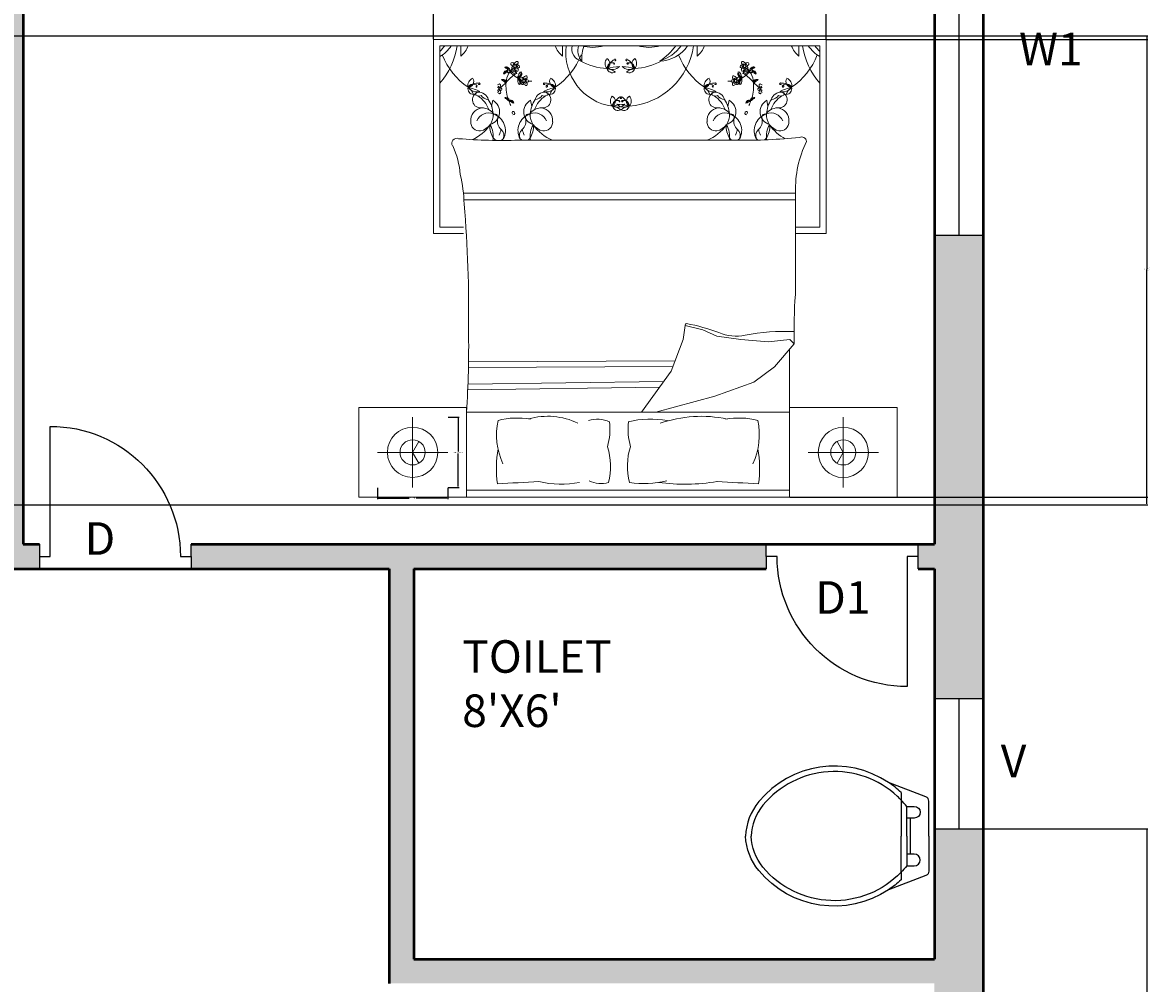
# Model space of a CAD drawing. Units: inches. Extents: x -15 to 420, y -514 to 86.
# Tile 7 of 8: x 212 to 420, y -251 to -74. Entities that reach past the tile are written whole.
import ezdxf

# ---------------------------------------------------------------- set-up
doc = ezdxf.new("R2010")
doc.units = ezdxf.units.IN
doc.header["$MEASUREMENT"] = 0
for name, color, linetype, lineweight in [('A-ANNO-DIMS', 2, 'Continuous', 18), ('A-ANNO-TEXT', 7, 'Continuous', 18), ('A-AREA-IDEN', 7, 'Continuous', 25), ('A-DOOR', 4, 'Continuous', 25), ('A-FLOR-FIXT', 9, 'Continuous', 25), ('A-FURN', 8, 'Continuous', 18), ('A-GLAZ', 41, 'Continuous', 25), ('A-WALL', 7, 'Continuous', 50), ('A-WALL-PATT', 8, 'Continuous', 13)]:
    doc.layers.add(name, color=color, linetype=linetype, lineweight=lineweight)
doc.styles.get("Standard").update_dxf_attribs({"font": 'arial.ttf'})
doc.dimstyles.get("Standard").update_dxf_attribs({"dimtxt": 0.18, "dimasz": 0.18, "dimexe": 0.18, "dimexo": 0.0625, "dimgap": 0.09, "dimtad": 0, "dimtih": 1, "dimtoh": 1, "dimdec": 0, "dimzin": 0, "dimdsep": 46, "dimlunit": 3, "dimtxsty": 'Standard', "dimcen": 0.09, "dimadec": 0, "dimazin": 0, "dimtfac": 1, "dimtdec": 0, "dimtofl": 0, "dimtmove": 0, "dimatfit": 3, "dimfxl": 1, "dimtolj": 1, "dimtzin": 0, "dimarcsym": 0})

# ---------------------------------------------------------------- blocks, each defined once
blk = doc.blocks.new('DOOR-SWING-24IN')
for p, q in [((26, 0), (26, 24)), ((2, 0), (0, 0)), ((28, 0), (26, 0))]:
    blk.add_line(p, q)
blk.add_arc((26, 0), 24, 90, 180)
blk = doc.blocks.new('WIN-W1-60IN')
for p, q in [((0, 60), (0, 0)), ((4.5, 60), (4.5, 0)), ((9, 0), (9, 60))]:
    blk.add_line(p, q)
blk = doc.blocks.new('VENT-V-24IN')
for p, q in [((0, 24), (0, 0)), ((4.5, 24), (4.5, 0)), ((9, 0), (9, 24))]:
    blk.add_line(p, q)
blk = doc.blocks.new('WC-PLAN')
for p, q in [((28.69, 20.98), (28.69, 19.56)), ((28.69, 19.56), (28.69, 12.91)), ((28.69, 6.26), (28.69, 12.91)), ((28.69, 6.26), (28.69, 4.85))]:
    blk.add_line(p, q)
for points in [[(26.37, 22.81, 0.383919), (2.44, 19.27, 0.163732), (0, 12.91, 0.359733)], [(28, 20.24, 0.431639), (3.21, 18.62, 0.162618), (1.01, 12.91, 0.470877)], [(28.69, 20.98, 0.040937), (26.37, 22.81, 0.163732)], [(33.8, 12.91), (33.8, 19.37, 0.31031), (33.26, 20.16), (26.37, 22.81, 0.209071)], [(28.69, 19.56, 0.014165), (28, 20.24, 0.162618)], [(29.71, 18.4, 0.022712), (28.69, 19.56, 0.162618)], [(29.71, 12.91), (29.71, 18.4, 0.022712)], [(29.71, 18.4), (31.12, 18.4, -1), (31.12, 16.24), (30.39, 16.24)], [(26.37, 3.02, -0.383919), (2.44, 6.56, -0.163732), (0, 12.91, -0.359733)], [(28.69, 6.26, -0.448546), (3.21, 7.2, -0.162618), (1.01, 12.91, -0.470877)], [(33.8, 12.91), (33.8, 6.46, -0.31031), (33.26, 5.67), (26.37, 3.02, -0.209071)], [(29.71, 12.91), (29.71, 7.43, -0.476108)], [(29.71, 7.43), (31.12, 7.43, 1), (31.12, 9.59), (30.39, 9.59)], [(29.71, 7.43, -0.022712), (28.69, 6.26, -0.162618)], [(28.69, 4.85, -0.040937), (26.37, 3.02, -0.163732)]]:
    blk.add_lwpolyline(points, format="xyb")
for points in [[(30.39, 16.24), (29.71, 16.24)], [(30.39, 9.59), (30.39, 16.24)], [(30.39, 9.59), (29.71, 9.59)]]:
    blk.add_lwpolyline(points)
blk = doc.blocks.new('BEDSIDE-LAMP-9-25IN')
for p, q in [((6.49, 12.97), (6.49, 0)), ((12.97, 6.49), (0, 6.49))]:
    blk.add_line(p, q)
for points in [[(6.49, 6.49), (7.64, 8.49)], [(6.49, 6.49), (7.64, 4.48)]]:
    blk.add_lwpolyline(points)
for radius in [4.63, 2.32]:
    blk.add_circle((6.49, 6.49), radius)
blk = doc.blocks.new('*D37')
at = {"layer": 'A-ANNO-DIMS', "color": 0, "lineweight": -2, "transparency": 16777216}
for p, q in [((290.77, -146.45), (292.83, -146.45)), ((292.65, -146.63), (292.65, -152.75)), ((292.65, -159.24), (292.65, -153.11)), ((290.77, -159.42), (292.83, -159.42))]:
    blk.add_line(p, q, dxfattribs=at)
at = {"layer": 'A-ANNO-DIMS', "color": 0, "transparency": 16777216}
for points in [[(292.62, -146.63), (292.68, -146.63), (292.65, -146.45)], [(292.62, -159.24), (292.68, -159.24), (292.65, -159.42)]]:
    blk.add_solid(points, dxfattribs=at)
at = {"layer": 'Defpoints', "color": 0, "transparency": 16777216}
for p in [(290.7, -146.45), (292.65, -146.45), (290.7, -159.42)]:
    blk.add_point(p, dxfattribs=at)
at = {"layer": 'A-ANNO-DIMS', "color": 0, "transparency": 16777216, "insert": (292.65, -152.93), "char_height": 0.18, "attachment_point": 5}
blk.add_mtext('\\A1;LAMP 1\'-1" TYP.', dxfattribs=at)
blk = doc.blocks.new('*D38')
at = {"layer": 'A-ANNO-DIMS', "color": 0, "lineweight": -2, "transparency": 16777216}
for p, q in [((277.73, -159.48), (277.73, -161.55)), ((290.7, -159.48), (290.7, -161.55)), ((277.91, -161.37), (283.59, -161.37)), ((290.52, -161.37), (284.85, -161.37))]:
    blk.add_line(p, q, dxfattribs=at)
at = {"layer": 'A-ANNO-DIMS', "color": 0, "transparency": 16777216}
for points in [[(277.91, -161.34), (277.91, -161.4), (277.73, -161.37)], [(290.52, -161.34), (290.52, -161.4), (290.7, -161.37)]]:
    blk.add_solid(points, dxfattribs=at)
at = {"layer": 'Defpoints', "color": 0, "transparency": 16777216}
for p in [(277.73, -159.42), (290.7, -159.42), (290.7, -161.37)]:
    blk.add_point(p, dxfattribs=at)
at = {"layer": 'A-ANNO-DIMS', "color": 0, "transparency": 16777216, "insert": (284.22, -161.37), "char_height": 0.18, "attachment_point": 5}
blk.add_mtext('\\A1;1\'-1" TYP.', dxfattribs=at)
blk = doc.blocks.new('*D62')
at = {"layer": 'A-ANNO-DIMS', "color": 0, "lineweight": -2, "transparency": 16777216}
for p, q in [((389.49, -222.38), (419.8, -222.38)), ((419.62, -222.56), (419.62, -272.45)), ((419.62, -322.7), (419.62, -272.81)), ((389.49, -322.88), (419.8, -322.88))]:
    blk.add_line(p, q, dxfattribs=at)
at = {"layer": 'A-ANNO-DIMS', "color": 0, "transparency": 16777216}
for points in [[(419.59, -222.56), (419.65, -222.56), (419.62, -222.38)], [(419.59, -322.7), (419.65, -322.7), (419.62, -322.88)]]:
    blk.add_solid(points, dxfattribs=at)
at = {"layer": 'Defpoints', "color": 0, "transparency": 16777216}
for p in [(389.42, -222.38), (419.62, -222.38), (389.42, -322.88)]:
    blk.add_point(p, dxfattribs=at)
at = {"layer": 'A-ANNO-DIMS', "color": 0, "transparency": 16777216, "insert": (419.62, -272.63), "char_height": 0.18, "attachment_point": 5}
blk.add_mtext('\\A1;8\'-4 1/2"', dxfattribs=at)
blk = doc.blocks.new('*D69')
at = {"layer": 'A-ANNO-DIMS', "color": 0, "lineweight": -2, "transparency": 16777216}
for p, q in [((141.76, -76.1), (419.8, -76.1)), ((419.62, -76.28), (419.62, -119.16)), ((419.62, -162.4), (419.62, -119.53)), ((134.84, -162.58), (419.8, -162.58))]:
    blk.add_line(p, q, dxfattribs=at)
at = {"layer": 'A-ANNO-DIMS', "color": 0, "transparency": 16777216}
for points in [[(419.59, -76.28), (419.65, -76.28), (419.62, -76.1)], [(419.59, -162.4), (419.65, -162.4), (419.62, -162.58)]]:
    blk.add_solid(points, dxfattribs=at)
at = {"layer": 'Defpoints', "color": 0, "transparency": 16777216}
for p in [(141.69, -76.1), (134.78, -162.58), (419.62, -162.58)]:
    blk.add_point(p, dxfattribs=at)
at = {"layer": 'A-ANNO-DIMS', "color": 0, "transparency": 16777216, "insert": (419.62, -119.34), "char_height": 0.18, "attachment_point": 5}
blk.add_mtext('\\A1;7\'-2 1/2"', dxfattribs=at)
blk = doc.blocks.new('*D70')
at = {"layer": 'A-ANNO-DIMS', "color": 0, "lineweight": -2, "transparency": 16777216}
for p, q in [((288.09, -76.72), (288.09, 43.5)), ((288.27, 43.32), (323.74, 43.32)), ((360.28, 43.32), (324.81, 43.32)), ((360.46, -76.72), (360.46, 43.5))]:
    blk.add_line(p, q, dxfattribs=at)
at = {"layer": 'A-ANNO-DIMS', "color": 0, "transparency": 16777216}
for points in [[(288.27, 43.35), (288.27, 43.29), (288.09, 43.32)], [(360.28, 43.35), (360.28, 43.29), (360.46, 43.32)]]:
    blk.add_solid(points, dxfattribs=at)
at = {"layer": 'Defpoints', "color": 0, "transparency": 16777216}
for p in [(360.46, 43.32), (288.09, -76.78), (360.46, -76.78)]:
    blk.add_point(p, dxfattribs=at)
at = {"layer": 'A-ANNO-DIMS', "color": 0, "transparency": 16777216, "insert": (324.27, 43.32), "char_height": 0.18, "attachment_point": 5}
blk.add_mtext('\\A1;6\'-0 1/2"', dxfattribs=at)
blk = doc.blocks.new('*D71')
at = {"layer": 'A-ANNO-DIMS', "color": 0, "lineweight": -2, "transparency": 16777216}
for p, q in [((360.53, -76.78), (419.8, -76.78)), ((419.62, -76.96), (419.62, -118.81)), ((419.62, -161.03), (419.62, -119.18)), ((353.77, -161.21), (419.8, -161.21))]:
    blk.add_line(p, q, dxfattribs=at)
at = {"layer": 'A-ANNO-DIMS', "color": 0, "transparency": 16777216}
for points in [[(419.59, -76.96), (419.65, -76.96), (419.62, -76.78)], [(419.59, -161.03), (419.65, -161.03), (419.62, -161.21)]]:
    blk.add_solid(points, dxfattribs=at)
at = {"layer": 'Defpoints', "color": 0, "transparency": 16777216}
for p in [(360.46, -76.78), (353.71, -161.21), (419.62, -161.21)]:
    blk.add_point(p, dxfattribs=at)
at = {"layer": 'A-ANNO-DIMS', "color": 0, "transparency": 16777216, "insert": (419.62, -118.99), "char_height": 0.18, "attachment_point": 5}
blk.add_mtext('\\A1;7\'-0 1/2"', dxfattribs=at)

msp = doc.modelspace()

# ---------------------------------------------------------------- hatches: boundary and pattern name
at = {"layer": 'A-WALL-PATT'}
h = msp.add_hatch(color=256, dxfattribs=at)
h.dxf.hatch_style = 1
h.paths.add_polyline_path([(266.67, -454.88), (240.92, -454.88), (240.92, -330.38), (236.42, -330.38), (236.42, -454.88), (218.42, -454.88), (218.42, -463.88), (266.67, -463.88)])
h.paths.add_polyline_path([(158.42, -454.88), (140.42, -454.88), (140.42, -394.88), (135.92, -394.88), (135.92, -454.88), (39.92, -454.88), (39.92, -412.88), (30.92, -412.88), (30.92, -463.88), (158.42, -463.88)])
h.paths.add_polyline_path([(39.92, -334.88), (135.92, -334.88), (135.92, -357.15), (140.42, -357.15), (140.42, -334.88), (173.95, -334.88), (173.95, -330.38), (39.92, -330.38), (39.92, -250.88), (155.51, -250.88), (155.51, -246.38), (140.42, -246.38), (140.42, -205.38), (138.17, -205.38), (135.92, -205.38), (135.92, -246.38), (39.92, -246.38), (39.92, -222.38), (30.92, -222.38), (30.92, -376.88), (39.92, -376.88)])
h.paths.add_polyline_path([(389.42, -382.88), (380.42, -382.88), (380.42, -454.88), (380.42, -463.88), (389.42, -463.88)])
h.paths.add_polyline_path([(352.42, -459.38), (352.42, -454.88), (326.67, -454.88), (326.67, -463.88), (352.42, -463.88)])
h.paths.add_polyline_path([(176.92, -169.88), (39.92, -169.88), (39.92, -112.88), (30.92, -112.88), (30.92, -198.38), (39.92, -198.38), (39.92, -174.38), (135.92, -174.38), (135.92, -177.38), (140.42, -177.38), (140.42, -174.38), (176.92, -174.38), (176.92, -172.13)])
h.paths.add_polyline_path([(39.92, 4.12), (93.92, 4.12), (93.92, 13.12), (30.92, 13.12), (30.92, -52.88), (39.92, -52.88)])
h.paths.add_polyline_path([(266.42, 13.12), (153.92, 13.12), (153.92, 4.12), (207.92, 4.12), (207.92, -169.88), (204.92, -169.88), (204.92, -174.38), (215.42, -174.38), (215.42, -169.88), (212.42, -169.88), (212.42, 4.12), (266.42, 4.12)])
h.paths.add_polyline_path([(389.42, 13.12), (326.42, 13.12), (326.42, 4.12), (380.42, 4.12), (380.42, -52.88), (389.42, -52.88)])
h.paths.add_polyline_path([(389.42, -112.88), (380.42, -112.88), (380.42, -169.88), (377.42, -169.88), (377.42, -174.38), (380.42, -174.38), (380.42, -198.38), (389.42, -198.38)])
h.paths.add_polyline_path([(349.42, -172.13), (349.42, -169.88), (243.42, -169.88), (243.42, -172.13), (243.42, -174.38), (279.92, -174.38), (279.92, -250.88), (380.42, -250.88), (380.42, -322.88), (389.42, -322.88), (389.42, -222.38), (380.42, -222.38), (380.42, -246.38), (284.42, -246.38), (284.42, -174.38), (349.42, -174.38)])

# ---------------------------------------------------------------- linework, layer by layer
at = {"layer": 'A-DOOR'}
for p, q in [((215.42, -169.88), (215.42, -174.38)), ((243.42, -172.13), (243.42, -169.88)), ((349.42, -172.13), (349.42, -169.88)), ((377.42, -174.38), (377.42, -169.88)), ((243.42, -172.13), (243.42, -174.38)), ((349.42, -172.13), (349.42, -174.38))]:
    msp.add_line(p, q, dxfattribs=at)
at = {"layer": 'A-FURN'}
for p, q in [((288.09, -76.78), (360.46, -76.78)), ((288.09, -112.54), (288.09, -76.78)), ((360.46, -76.78), (360.46, -112.54)), ((289.24, -77.93), (289.24, -111.39)), ((359.31, -77.93), (289.24, -77.93)), ((359.31, -111.39), (359.31, -77.93)), ((299.02, -88), (298.8, -89.12)), ((305.96, -88), (306.18, -89.12)), ((342.59, -88), (342.37, -89.12)), ((349.53, -88), (349.75, -89.12)), ((303.77, -95.36), (344.08, -95.36)), ((293.6, -105.11), (354.85, -105.11)), ((293.7, -106.35), (354.85, -106.35)), ((289.24, -111.39), (293.61, -111.39)), ((354.85, -111.39), (359.31, -111.39)), ((293.59, -112.54), (288.09, -112.54)), ((360.46, -112.54), (354.85, -112.54)), ((334.09, -132.12), (334.49, -129.51)), ((334.49, -129.51), (337.71, -130.31)), ((337.71, -130.31), (340.32, -131.52)), ((331.88, -137.95), (334.09, -132.12)), ((340.32, -131.52), (344.75, -132.12)), ((344.75, -132.12), (349.77, -132.52)), ((349.77, -132.52), (353.8, -132.12)), ((354.6, -132.92), (350.98, -137.14)), ((353.8, -132.12), (354.6, -132.92)), ((353.71, -161.21), (353.71, -133.96)), ((294.5, -136.23), (332.59, -136.07)), ((294.5, -137.25), (332.2, -137.1)), ((326.44, -145.52), (331.88, -137.95)), ((350.98, -137.14), (347.16, -139.96)), ((294.41, -141.39), (329.76, -140.9)), ((294.45, -140.38), (330.5, -139.87)), ((347.16, -139.96), (339.92, -142.57)), ((339.92, -142.57), (329.1, -145.52)), ((353.71, -145.52), (294.15, -145.52)), ((294.15, -159.93), (353.71, -159.93)), ((373.57, -161.21), (274.29, -161.21))]:
    msp.add_line(p, q, dxfattribs=at)
for points in [[(293.72, -107.13, 0.056112), (293, -101.67, 0.095341), (291.61, -96.41)], [(354.81, -123.83, 0.001242), (354.85, -105, -0.127202), (356.85, -95.61)], [(299.85, -158.73, -0.074897), (299.97, -152.25, 0.472817)], [(320.15, -151.89, -0.14099), (320.35, -158.5, -0.235245)], [(324.39, -151.89, 0.14099), (324.2, -158.5, 0.235245)], [(348.01, -158.73, 0.074897), (347.89, -152.25, -0.472817)]]:
    msp.add_lwpolyline(points, format="xyb", dxfattribs=at)
for points in [[(294.15, -161.21), (294.15, -144.66), (274.29, -144.66), (274.29, -161.21)], [(353.71, -144.66), (373.57, -144.66), (373.57, -161.21)]]:
    msp.add_lwpolyline(points, dxfattribs=at)
for centre in [(303.1, -81.73), (345.45, -81.73), (304.76, -84.4), (343.79, -84.4)]:
    msp.add_circle(centre, 0.253, dxfattribs=at)
for centre, radius, start, end in [((286.09, -74.45), 6.32, 299.8884, 326.5383), ((283.82, -73.27), 7.87, 313.5186, 323.6964), ((279.59, -76.18), 12.96, 318.1144, 352.255), ((289.63, -75.91), 5.27, 311.0454, 337.4453), ((275.19, -78.74), 17.94, 356.3481, 2.5919), ((315.35, -75.91), 5.27, 202.5547, 228.9546), ((329.79, -78.74), 17.94, 177.4081, 183.6519), ((322.5, -79.18), 10.03, 172.8636, 261.8197), ((315.88, -78.48), 2.33, 166.3898, 259.0739), ((317.63, -78.8), 2.94, 162.8609, 221.9049), ((317.47, -71.11), 7.13, 252.9798, 286.4569), ((321.21, -80.09), 5.8, 158.117, 186.6195), ((320.29, -67.44), 10.54, 264.3643, 265.6213), ((325.84, -60.22), 18.84, 250.0972, 250.2783), ((323.16, -76.18), 12.96, 274.4623, 352.255), ((327.77, -71.11), 7.13, 253.5431, 287.0202), ((324.95, -67.44), 10.54, 274.3787, 275.6357), ((319.4, -60.22), 18.84, 289.7217, 289.9028), ((329.66, -74.45), 6.32, 271.272, 326.5383), ((323.25, -71.06), 11.71, 304.0123, 324.053), ((327.39, -73.27), 7.87, 287.8504, 323.6964), ((318.76, -78.74), 17.94, 356.3481, 2.5919), ((333.2, -75.91), 5.27, 311.0454, 337.4453), ((358.92, -75.91), 5.27, 202.5547, 228.9546), ((373.36, -78.74), 17.94, 177.4081, 183.6519), ((368.96, -76.18), 12.96, 187.745, 221.8856), ((362.46, -74.45), 6.32, 213.4617, 240.1116), ((364.73, -73.27), 7.87, 216.3036, 226.4814), ((301.77, -74.9), 12.96, 201.4092, 235.6135), ((303.45, -81.27), 0.417, 100.9597, 208.7804), ((303.09, -81.04), 0.588, 291.6382, 4.947), ((303.49, -81.01), 0.194, 4.947, 127.5263), ((303.21, -74.9), 12.96, 304.3865, 338.5908), ((321.09, -69.24), 12.96, 242.5854, 265.5377), ((321.15, -81.2), 1.44, 140.8855, 222.2127), ((319.51, -81.24), 1.08, 301.6373, 61.4609), ((323.18, -83.23), 3.28, 121.989, 161.0841), ((321.53, -80.58), 0.161, 288.4408, 121.989), ((321.56, -80.66), 0.0782, 171.9833, 288.4408), ((323.71, -80.58), 0.161, 58.011, 251.5592), ((323.68, -80.66), 0.0782, 251.5592, 8.0167), ((322.06, -83.23), 3.28, 18.9159, 58.011), ((325.73, -81.24), 1.08, 118.5391, 238.3627), ((324.09, -81.2), 1.44, 317.7873, 39.1145), ((324.15, -69.24), 12.96, 274.4623, 297.4146), ((345.34, -74.9), 12.96, 201.4092, 235.6135), ((345.06, -81.01), 0.194, 52.4737, 175.053), ((345.46, -81.04), 0.588, 175.053, 248.3618), ((345.1, -81.27), 0.417, 331.2196, 79.0403), ((346.78, -74.9), 12.96, 304.3865, 338.5908), ((301.26, -83.03), 0.282, 123.0979, 213.1364), ((301.75, -83.43), 0.764, 92.3172, 160.5201), ((305.24, -89.24), 7.39, 121.1156, 124.8118), ((301.66, -83.15), 0.658, 82.6008, 147.1845), ((301.47, -82.1), 0.282, 55.6077, 145.6462), ((301.28, -82.71), 0.764, 21.7087, 93.0299), ((297.25, -88.16), 7.39, 53.6254, 57.3216), ((301.58, -83.17), 0.292, 45.7354, 121.1156), ((305.56, -85.03), 4.12, 150.7959, 175.244), ((311.49, -93.81), 13.56, 127.8256, 137.7588), ((301.51, -82.52), 0.658, 342.8042, 79.6943), ((301.46, -82.45), 0.292, 338.2452, 53.6254), ((301.93, -82.64), 0.221, 158.2452, 340.6395), ((301.93, -82.8), 0.221, 225.7354, 48.1297), ((306.08, -80.79), 4.4, 201.7087, 206.2181), ((302.58, -83.8), 1.15, 40.9365, 112.7695), ((302.2, -83.41), 0.678, 49.3812, 95.5456), ((305.56, -85.03), 4.12, 137.5083, 145.9967), ((302.69, -83.15), 0.7, 61.1838, 141.6792), ((305.98, -79.56), 4.94, 220.182, 239.456), ((302.57, -81.26), 0.25, 134.3732, 211.9501), ((303.03, -80.97), 0.797, 211.9501, 255.2442), ((302.59, -81.54), 0.499, 8.5614, 112.5914), ((302.82, -82.08), 0.345, 88.5719, 233.8954), ((302.78, -82.18), 0.248, 228.2946, 6.2474), ((303.17, -82.28), 0.815, 229.3812, 289.9959), ((302.73, -81.52), 0.167, 352.868, 97.094), ((302.55, -81.88), 0.348, 298.8493, 359.9355), ((302.63, -82.18), 0.398, 4.2123, 48.1587), ((303.45, -82.12), 0.422, 183.635, 258.4363), ((302.64, -83.27), 0.837, 15.6484, 62.2957), ((303.4, -81.97), 0.241, 178.1325, 268.8919), ((303.9, -81.82), 0.768, 132.3896, 156.5724), ((303.56, -81.92), 0.414, 42.3208, 130.2111), ((303.65, -81.49), 0.523, 226.3462, 279.6513), ((303.11, -82.46), 0.608, 7.4968, 71.2737), ((303.55, -80.94), 0.828, 254.2829, 276.9148), ((303.53, -82.43), 0.195, 215.0752, 14.7644), ((303.12, -82.73), 1.15, 287.889, 359.722), ((303.7, -81.79), 0.218, 279.6513, 42.3208), ((304.56, -83.5), 0.815, 110.6625, 171.2773), ((303.51, -83.09), 0.837, 338.3627, 25.0101), ((321.14, -82.12), 1.06, 76.148, 182.2415), ((322.8, -90.82), 9.07, 92.7418, 107.407), ((320.93, -80.3), 2.05, 245.6899, 314.4589), ((320.03, -84.38), 2.21, 44.6273, 88.5415), ((321.11, -81.86), 1.07, 196.1963, 296.9726), ((321.38, -81.28), 0.0845, 140.1909, 76.0209), ((322.44, -90.82), 9.07, 72.593, 87.2582), ((324.31, -80.3), 2.05, 225.5411, 294.3101), ((325.21, -84.38), 2.21, 91.4585, 135.3727), ((324.13, -81.86), 1.07, 243.0274, 343.8037), ((323.88, -81.23), 0.14, 103.852, 39.9245), ((324.1, -82.12), 1.06, 357.7585, 103.852), ((345.04, -83.09), 0.837, 154.9899, 201.6373), ((345.43, -82.73), 1.15, 180.278, 252.111), ((343.99, -83.5), 0.815, 8.7227, 69.3375), ((344.85, -81.79), 0.218, 137.6792, 260.3487), ((344.99, -81.92), 0.414, 49.7889, 137.6792), ((344.9, -81.49), 0.523, 260.3487, 313.6538), ((345.44, -82.46), 0.608, 108.7263, 172.5032), ((345.02, -82.43), 0.195, 165.2356, 324.9248), ((345, -80.94), 0.828, 263.0852, 285.7171), ((342.57, -79.56), 4.94, 300.544, 319.818), ((345.91, -83.27), 0.837, 117.7043, 164.3516), ((345.97, -83.8), 1.15, 67.2305, 139.0635), ((345.38, -82.28), 0.815, 250.0041, 310.6188), ((345.15, -81.97), 0.241, 271.1081, 1.8675), ((344.65, -81.82), 0.768, 23.4276, 47.6104), ((345.1, -82.12), 0.422, 281.5637, 356.365), ((337.06, -93.81), 13.56, 42.2412, 52.1744), ((345.96, -81.54), 0.499, 67.4086, 171.4386), ((345.92, -82.18), 0.398, 131.8413, 175.7877), ((345.76, -82.18), 0.248, 173.7526, 311.7054), ((345.86, -83.15), 0.7, 38.3208, 118.8162), ((345.82, -81.52), 0.167, 82.906, 187.132), ((346, -81.88), 0.348, 180.0645, 241.1507), ((345.52, -80.97), 0.797, 284.7558, 328.0499), ((345.73, -82.08), 0.345, 306.1046, 91.4281), ((346.35, -83.41), 0.678, 84.4544, 130.6188), ((342.99, -85.03), 4.12, 34.0033, 42.4917), ((345.98, -81.26), 0.25, 328.0499, 45.6268), ((347.04, -82.52), 0.658, 100.3057, 197.1958), ((346.61, -82.8), 0.221, 131.8703, 314.2646), ((346.62, -82.64), 0.221, 199.3605, 21.7548), ((342.47, -80.79), 4.4, 333.7819, 338.2913), ((347.27, -82.71), 0.764, 86.9701, 158.2913), ((342.99, -85.03), 4.12, 4.756, 29.2041), ((346.97, -83.17), 0.292, 58.8844, 134.2646), ((347.09, -82.45), 0.292, 126.3746, 201.7548), ((346.89, -83.15), 0.658, 32.8155, 97.3992), ((346.8, -83.43), 0.764, 19.4799, 87.6828), ((347.08, -82.1), 0.282, 34.3538, 124.3923), ((351.3, -88.16), 7.39, 122.6784, 126.3746), ((343.31, -89.24), 7.39, 55.1882, 58.8844), ((347.29, -83.03), 0.282, 326.8636, 56.9021), ((295.85, -85.29), 1.44, 110.9613, 192.2885), ((294.41, -84.52), 1.08, 271.7131, 31.5367), ((296.6, -88.07), 3.28, 92.0648, 131.1598), ((295.38, -86.09), 1.06, 46.2238, 152.3173), ((296.47, -85.03), 0.0782, 142.0591, 258.5166), ((296.49, -84.95), 0.161, 258.5166, 92.0648), ((300.2, -85.43), 0.417, 100.9597, 142.2379), ((299.85, -85.21), 0.588, 291.6382, 4.947), ((300.24, -85.18), 0.194, 4.947, 127.5263), ((294.58, -78.24), 9.43, 307.9541, 316.8459), ((300.7, -86.96), 2.8, 82.8698, 91.6736), ((301.09, -83.94), 0.521, 205.5379, 258.6744), ((300.34, -85.71), 1.57, 59.344, 79.7412), ((300, -85.7), 1.6, 43.6929, 51.7899), ((300.98, -84.66), 0.476, 355.7131, 81.6568), ((300.71, -85.07), 0.832, 27.3659, 59.344), ((301.34, -84.52), 0.202, 202.5583, 304.2343), ((309.66, -85.24), 8.22, 176.1723, 196.4158), ((303.08, -83.27), 0.678, 305.1128, 351.2773), ((303.44, -84.52), 0.7, 3.8774, 87.1501), ((302.94, -84.24), 0.678, 352.0748, 38.2393), ((302.82, -84.77), 1.15, 343.6301, 55.4631), ((304.42, -84.45), 0.815, 172.0748, 232.6895), ((303.64, -83.15), 0.7, 271.4625, 339.4747), ((303.3, -84.54), 0.837, 318.342, 4.9894), ((304.22, -83.92), 0.25, 134.3732, 211.9501), ((305.98, -79.56), 4.94, 246.1523, 246.9499), ((304.69, -83.63), 0.797, 211.9501, 255.2442), ((304.24, -84.21), 0.499, 8.5614, 112.5914), ((304.48, -84.75), 0.345, 88.5719, 233.8954), ((304.44, -84.84), 0.248, 228.2946, 6.2474), ((304.38, -84.18), 0.167, 352.868, 97.094), ((304.21, -84.55), 0.348, 298.8493, 359.9355), ((304.29, -84.85), 0.398, 4.2123, 48.1587), ((305.1, -83.93), 0.417, 100.9597, 208.7804), ((305.11, -84.79), 0.422, 183.635, 258.4363), ((305.05, -84.64), 0.241, 178.1325, 268.8919), ((305.55, -84.49), 0.768, 132.3896, 156.5724), ((305.21, -84.58), 0.414, 42.3208, 130.2111), ((305.31, -84.15), 0.523, 226.3462, 279.6513), ((304.75, -83.71), 0.588, 291.6382, 4.947), ((304.77, -85.12), 0.608, 7.4968, 71.2737), ((305.21, -83.61), 0.828, 254.2829, 276.9148), ((305.14, -83.67), 0.194, 4.947, 127.5263), ((305.18, -85.09), 0.195, 215.0752, 14.7644), ((305.36, -84.45), 0.218, 279.6513, 42.3208), ((305.98, -79.56), 4.94, 265.2415, 272.8929), ((308.49, -84.95), 0.161, 87.9352, 281.4834), ((308.38, -88.07), 3.28, 48.8402, 87.9352), ((308.51, -85.03), 0.0782, 281.4834, 37.9409), ((309.6, -86.09), 1.06, 27.6827, 133.7762), ((310.57, -84.52), 1.08, 148.4633, 268.2869), ((309.13, -85.29), 1.44, 347.7115, 69.0387), ((339.42, -85.29), 1.44, 110.9613, 192.2885), ((337.98, -84.52), 1.08, 271.7131, 31.5367), ((340.17, -88.07), 3.28, 92.0648, 131.1598), ((338.95, -86.09), 1.06, 46.2238, 152.3173), ((340.04, -85.03), 0.0782, 142.0591, 258.5166), ((340.06, -84.95), 0.161, 258.5166, 92.0648), ((342.57, -79.56), 4.94, 267.1071, 274.7585), ((343.19, -84.45), 0.218, 137.6792, 260.3487), ((343.34, -84.58), 0.414, 49.7889, 137.6792), ((343.24, -84.15), 0.523, 260.3487, 313.6538), ((343.37, -85.09), 0.195, 165.2356, 324.9248), ((343.78, -85.12), 0.608, 108.7263, 172.5032), ((343.41, -83.67), 0.194, 52.4737, 175.053), ((343.8, -83.71), 0.588, 175.053, 248.3618), ((343.34, -83.61), 0.828, 263.0852, 285.7171), ((343.5, -84.64), 0.241, 271.1081, 1.8675), ((343, -84.49), 0.768, 23.4276, 47.6104), ((343.45, -83.93), 0.417, 331.2196, 79.0403), ((343.44, -84.79), 0.422, 281.5637, 356.365), ((344.31, -84.21), 0.499, 67.4086, 171.4386), ((344.11, -84.84), 0.248, 173.7526, 311.7054), ((344.26, -84.85), 0.398, 131.8413, 175.7877), ((344.17, -84.18), 0.167, 82.906, 187.132), ((344.34, -84.55), 0.348, 180.0645, 241.1507), ((343.86, -83.63), 0.797, 284.7558, 328.0499), ((344.07, -84.75), 0.345, 306.1046, 91.4281), ((344.91, -83.15), 0.7, 200.5253, 268.5375), ((345.11, -84.52), 0.7, 92.8499, 176.1226), ((345.25, -84.54), 0.837, 175.0106, 221.658), ((344.33, -83.92), 0.25, 328.0499, 45.6268), ((342.57, -79.56), 4.94, 293.0501, 293.8477), ((345.73, -84.77), 1.15, 124.5369, 196.3699), ((344.13, -84.45), 0.815, 307.3105, 7.9252), ((345.47, -83.27), 0.678, 188.7227, 234.8872), ((345.61, -84.24), 0.678, 141.7607, 187.9252), ((338.89, -85.24), 8.22, 343.5842, 3.8277), ((347.57, -84.66), 0.476, 98.3432, 184.2869), ((347.84, -85.07), 0.832, 120.656, 152.6341), ((347.21, -84.52), 0.202, 235.7657, 337.4417), ((353.97, -78.24), 9.43, 223.1541, 232.0459), ((348.55, -85.7), 1.6, 128.2101, 136.3071), ((348.21, -85.71), 1.57, 100.2588, 120.656), ((347.85, -86.96), 2.8, 88.3264, 97.1302), ((347.46, -83.94), 0.521, 281.3256, 334.4621), ((348.31, -85.18), 0.194, 52.4737, 175.053), ((348.7, -85.21), 0.588, 175.053, 248.3618), ((348.35, -85.43), 0.417, 37.7621, 79.0403), ((352.06, -84.95), 0.161, 87.9352, 281.4834), ((351.95, -88.07), 3.28, 48.8402, 87.9352), ((352.08, -85.03), 0.0782, 281.4834, 37.9409), ((353.17, -86.09), 1.06, 27.6827, 133.7762), ((354.14, -84.52), 1.08, 148.4633, 268.2869), ((352.7, -85.29), 1.44, 347.7115, 69.0387), ((295.49, -85.86), 1.07, 166.272, 267.0484), ((292.48, -94.45), 9.07, 62.8176, 77.4827), ((296.11, -84.4), 2.05, 215.7657, 284.5347), ((293.29, -87.49), 2.21, 14.7031, 58.6173), ((296.75, -87.91), 1.49, 109.1312, 279.736), ((296.44, -86.3), 0.913, 216.7319, 296.0245), ((296, -85.48), 0.0845, 110.2667, 46.2271), ((293.8, -91.19), 4.69, 18.2955, 58.7386), ((296.39, -88.36), 1.86, 15.6955, 94.031), ((298.4, -85.89), 1.98, 218.4175, 263.8338), ((299.85, -85.9), 0.253, 273.2768, 86.7232), ((300.2, -86.29), 0.422, 217.3642, 258.4363), ((300.15, -86.14), 0.241, 178.1325, 268.8919), ((300.65, -85.99), 0.768, 132.3896, 156.5724), ((300.31, -86.09), 0.414, 42.3208, 130.2111), ((300.41, -85.65), 0.523, 226.3462, 279.6513), ((299.87, -86.62), 0.608, 7.4968, 71.2737), ((300.31, -85.11), 0.828, 254.2829, 276.9148), ((300.28, -86.59), 0.195, 215.0752, 14.7644), ((300.46, -85.95), 0.218, 279.6513, 42.3208), ((311.18, -91.19), 4.69, 121.2614, 161.7045), ((308.59, -88.36), 1.86, 85.969, 164.3045), ((306.58, -85.89), 1.98, 276.1662, 321.5825), ((308.23, -87.91), 1.49, 260.264, 70.8688), ((308.54, -86.3), 0.913, 243.9755, 323.2681), ((308.87, -84.4), 2.05, 255.4653, 324.2343), ((312.5, -94.45), 9.07, 102.5173, 117.1824), ((308.96, -85.43), 0.14, 133.7762, 69.7183), ((309.49, -85.86), 1.07, 272.9516, 13.728), ((311.69, -87.49), 2.21, 121.3827, 165.2969), ((322.14, -88.14), 1.44, 140.8855, 222.2127), ((320.51, -88.19), 1.08, 301.6373, 61.4609), ((324.73, -88.19), 1.08, 118.5391, 238.3627), ((323.1, -88.14), 1.44, 317.7873, 39.1145), ((339.06, -85.86), 1.07, 166.272, 267.0484), ((336.86, -87.49), 2.21, 14.7031, 58.6173), ((339.68, -84.4), 2.05, 215.7657, 284.5347), ((336.05, -94.45), 9.07, 62.8176, 77.4827), ((340.32, -87.91), 1.49, 109.1312, 279.736), ((340.01, -86.3), 0.913, 216.7319, 296.0245), ((339.57, -85.48), 0.0845, 110.2667, 46.2271), ((337.37, -91.19), 4.69, 18.2955, 58.7386), ((339.96, -88.36), 1.86, 15.6955, 94.031), ((341.97, -85.89), 1.98, 218.4175, 263.8338), ((348.09, -85.95), 0.218, 137.6792, 260.3487), ((348.24, -86.09), 0.414, 49.7889, 137.6792), ((348.14, -85.65), 0.523, 260.3487, 313.6538), ((348.27, -86.59), 0.195, 165.2356, 324.9248), ((348.68, -86.62), 0.608, 108.7263, 172.5032), ((348.24, -85.11), 0.828, 263.0852, 285.7171), ((348.4, -86.14), 0.241, 271.1081, 1.8675), ((347.9, -85.99), 0.768, 23.4276, 47.6104), ((348.35, -86.29), 0.422, 281.5637, 322.6358), ((348.7, -85.9), 0.253, 93.2768, 266.7232), ((354.75, -91.19), 4.69, 121.2614, 161.7045), ((352.16, -88.36), 1.86, 85.969, 164.3045), ((350.15, -85.89), 1.98, 276.1662, 321.5825), ((351.8, -87.91), 1.49, 260.264, 70.8688), ((352.11, -86.3), 0.913, 243.9755, 323.2681), ((356.07, -94.45), 9.07, 102.5173, 117.1824), ((352.44, -84.4), 2.05, 255.4653, 324.2343), ((352.53, -85.43), 0.14, 133.7762, 69.7183), ((355.26, -87.49), 2.21, 121.3827, 165.2969), ((353.06, -85.86), 1.07, 272.9516, 13.728), ((293.75, -90.82), 5.33, 3.4924, 33.7117), ((297.79, -90.13), 2.47, 286.8663, 60.0915), ((301.29, -90.3), 2.8, 82.8698, 91.6736), ((301.68, -87.28), 0.521, 205.5379, 258.6744), ((300.93, -89.05), 1.57, 59.344, 79.7412), ((300.59, -89.04), 1.6, 43.6929, 51.7899), ((301.57, -88), 0.476, 355.7131, 81.6568), ((301.3, -88.41), 0.832, 27.3659, 59.344), ((301.93, -87.86), 0.202, 202.5583, 304.2343), ((309.66, -85.24), 8.22, 200.1059, 206.9968), ((302.3, -88.43), 0.476, 36.5232, 122.4668), ((302.05, -88.86), 0.832, 58.836, 90.8141), ((302.24, -88.05), 0.202, 173.9457, 275.6216), ((301.84, -89.79), 1.6, 66.3901, 74.4871), ((302.88, -88), 0.521, 219.5056, 272.6421), ((301.67, -89.49), 1.57, 38.4388, 58.836), ((300.4, -89.77), 2.8, 26.5064, 35.3102), ((307.19, -90.13), 2.47, 119.9085, 253.1337), ((311.23, -90.82), 5.33, 146.2883, 176.5076), ((322.13, -89.07), 1.06, 76.148, 182.2415), ((324.18, -90.17), 3.28, 121.989, 161.0841), ((321.92, -87.24), 2.05, 245.6899, 314.4589), ((323.79, -97.76), 9.07, 92.7418, 107.407), ((322.11, -88.81), 1.07, 196.1963, 296.9726), ((321.02, -91.32), 2.21, 44.6273, 88.5415), ((323.32, -87.24), 2.05, 225.5411, 294.3101), ((321.45, -97.76), 9.07, 72.593, 87.2582), ((322.37, -88.23), 0.0845, 140.1909, 76.0209), ((322.53, -87.53), 0.161, 288.4408, 121.989), ((322.55, -87.61), 0.0782, 171.9833, 288.4408), ((322.72, -87.53), 0.161, 58.011, 251.5592), ((323.13, -88.81), 1.07, 243.0274, 343.8037), ((324.22, -91.32), 2.21, 91.4585, 135.3727), ((322.69, -87.61), 0.0782, 251.5592, 8.0167), ((322.89, -88.17), 0.14, 103.852, 39.9245), ((321.06, -90.17), 3.28, 18.9159, 58.011), ((323.11, -89.07), 1.06, 357.7585, 103.852), ((337.32, -90.82), 5.33, 3.4924, 33.7117), ((341.36, -90.13), 2.47, 286.8663, 60.0915), ((346.88, -89.49), 1.57, 121.164, 141.5612), ((348.15, -89.77), 2.8, 144.6898, 153.4936), ((345.67, -88), 0.521, 267.3579, 320.4944), ((346.25, -88.43), 0.476, 57.5332, 143.4768), ((346.49, -88.86), 0.832, 89.1859, 121.164), ((346.71, -89.79), 1.6, 105.5129, 113.6099), ((338.89, -85.24), 8.22, 333.0032, 339.8941), ((346.31, -88.05), 0.202, 264.3784, 6.0543), ((346.98, -88), 0.476, 98.3432, 184.2869), ((347.25, -88.41), 0.832, 120.656, 152.6341), ((346.62, -87.86), 0.202, 235.7657, 337.4417), ((347.96, -89.04), 1.6, 128.2101, 136.3071), ((347.62, -89.05), 1.57, 100.2588, 120.656), ((347.26, -90.3), 2.8, 88.3264, 97.1302), ((346.87, -87.28), 0.521, 281.3256, 334.4621), ((350.76, -90.13), 2.47, 119.9085, 253.1337), ((354.8, -90.82), 5.33, 146.2883, 176.5076), ((297.3, -91.74), 2.37, 97.1143, 185.0551), ((298.23, -92.64), 2.3, 68.5779, 158.4181), ((296.09, -90.74), 2.99, 283.079, 4.7067), ((296.88, -92.26), 2.88, 35.9599, 87.6409), ((302.3, -92.84), 3.83, 143.6555, 147.2989), ((299.35, -91.17), 0.616, 344.8529, 102.6959), ((298.17, -93.56), 3.16, 330.8249, 70.7178), ((301.91, -91.87), 2.04, 164.8529, 228.4347), ((302.77, -90.24), 0.191, 79.5616, 257.2949), ((302.75, -90.36), 0.311, 259.5864, 79.5616), ((306.81, -93.56), 3.16, 109.2822, 209.1751), ((303.07, -91.87), 2.04, 311.5653, 15.1471), ((305.63, -91.17), 0.616, 77.3041, 195.1471), ((308.1, -92.26), 2.88, 92.3591, 144.0401), ((302.68, -92.84), 3.83, 32.7011, 36.3445), ((308.89, -90.74), 2.99, 175.2933, 256.921), ((306.75, -92.64), 2.3, 21.5819, 111.4221), ((307.68, -91.74), 2.37, 354.9449, 82.8857), ((340.87, -91.74), 2.37, 97.1143, 185.0551), ((341.8, -92.64), 2.3, 68.5779, 158.4181), ((339.66, -90.74), 2.99, 283.079, 4.7067), ((340.45, -92.26), 2.88, 35.9599, 87.6409), ((345.87, -92.84), 3.83, 143.6555, 147.2989), ((342.92, -91.17), 0.616, 344.8529, 102.6959), ((341.74, -93.56), 3.16, 330.8249, 70.7178), ((345.48, -91.87), 2.04, 164.8529, 228.4347), ((345.8, -90.36), 0.311, 100.4384, 280.4136), ((345.78, -90.24), 0.191, 282.7051, 100.4384), ((350.38, -93.56), 3.16, 109.2822, 209.1751), ((346.64, -91.87), 2.04, 311.5653, 15.1471), ((349.2, -91.17), 0.616, 77.3041, 195.1471), ((351.67, -92.26), 2.88, 92.3591, 144.0401), ((346.25, -92.84), 3.83, 32.7011, 36.3445), ((352.46, -90.74), 2.99, 175.2933, 256.921), ((350.32, -92.64), 2.3, 21.5819, 111.4221), ((351.25, -91.74), 2.37, 354.9449, 82.8857), ((296.61, -91.98), 1.68, 178.9462, 275.5144), ((292.23, -88.37), 7.51, 293.6453, 326.3329), ((302.3, -92.84), 3.83, 175.2696, 214.215), ((294.99, -94.63), 4.11, 349.249, 31.1782), ((297.69, -92.98), 2.85, 330.0851, 352.564), ((299.58, -94.5), 1.49, 336.1646, 48.4347), ((305.4, -94.5), 1.49, 131.5653, 203.8354), ((307.28, -92.98), 2.85, 187.436, 209.9149), ((302.68, -92.84), 3.83, 325.785, 4.7304), ((309.99, -94.63), 4.11, 148.8218, 190.2867), ((312.75, -88.37), 7.51, 213.6671, 248.5059), ((308.37, -91.98), 1.68, 264.4856, 1.0538), ((340.18, -91.98), 1.68, 178.9462, 275.5144), ((335.8, -88.37), 7.51, 291.4941, 326.3329), ((345.87, -92.84), 3.83, 175.2696, 214.215), ((338.56, -94.63), 4.11, 349.7133, 31.1782), ((341.27, -92.98), 2.85, 330.0851, 352.564), ((343.15, -94.5), 1.49, 336.1646, 48.4347), ((348.97, -94.5), 1.49, 131.5653, 203.8354), ((350.85, -92.98), 2.85, 187.436, 209.9149), ((346.25, -92.84), 3.83, 325.785, 4.7304), ((353.56, -94.63), 4.11, 148.8218, 189.1554), ((356.32, -88.37), 7.51, 213.6671, 243.2997), ((351.94, -91.98), 1.68, 264.4856, 1.0538), ((292.36, -95.91), 0.905, 66.5219, 213.8264), ((300.73, 1.19), 96.6, 265.2402, 271.8035), ((300.08, -94.26), 1.2, 217.675, 252.5814), ((300.08, -94.26), 1.2, 286.6343, 315.5483), ((304.9, -94.26), 1.2, 224.4517, 246.7144), ((304.9, -94.26), 1.2, 293.2856, 322.325), ((343.65, -94.26), 1.2, 217.675, 246.7144), ((345.27, 7.98), 103.35, 269.3433, 275.6887), ((343.65, -94.26), 1.2, 293.229, 315.5483), ((348.47, -94.26), 1.2, 224.4517, 243.558), ((348.47, -94.26), 1.2, 300.0293, 322.325), ((355.93, -95.67), 0.916, 3.98, 117.3412), ((61.87, -126.9), 232.69, 359.1145, 4.8735), ((445.62, -130.45), 91.06, 175.8294, 181.553), ((116.18, -133.39), 178.38, 356.1, 0.9282), ((334.72, -129.43), 0.24, 88.8623, 199.7536), ((327.6, -167.02), 38.5, 70.1194, 79.3383), ((343.95, -123.42), 8.08, 246.2616, 281.3392), ((352.9, -168.08), 37.47, 87.4519, 101.3392), ((312.5, -149.64), 12.8, 168.2417, 204.8684), ((303.39, -159.89), 13.3, 78.9631, 104.8961), ((309.13, -158.91), 12.64, 63.8761, 106.1746), ((318.33, -152.07), 5.26, 65.0183, 108.5407), ((308.45, -148.57), 12.16, 344.1707, 5.9871), ((336.1, -148.57), 12.16, 174.0129, 195.8293), ((328.12, -164.31), 17.51, 79.8617, 103.6238), ((337.46, -169.35), 23.07, 78.0397, 109.2615), ((344.47, -159.89), 13.3, 75.1039, 101.0369), ((335.36, -149.64), 12.8, 335.1316, 11.7583), ((354.57, -1103.5), 946.35, 92.85022, 93.31479), ((311.63, -141.36), 17.45, 256.3427, 281.1841), ((318.99, -153.78), 4.91, 243.3437, 286.1026), ((326.8, -141), 17.69, 261.5249, 283.96), ((334.41, -122.81), 36, 262.2196, 279.497), ((293.29, -1103.5), 946.35, 86.68521, 87.14978)]:
    msp.add_arc(centre, radius, start, end, dxfattribs=at)
at = {"layer": 'A-GLAZ'}
for p, q in [((380.42, -112.88), (389.42, -112.88)), ((389.42, -198.38), (380.42, -198.38)), ((380.42, -222.38), (389.42, -222.38))]:
    msp.add_line(p, q, dxfattribs=at)
at = {"layer": 'A-WALL'}
for p, q in [((389.42, 13.12), (389.42, -463.88)), ((212.42, 4.12), (212.42, -169.88)), ((380.42, 4.12), (380.42, -169.88)), ((212.42, -169.88), (215.42, -169.88)), ((243.42, -169.88), (380.42, -169.88)), ((140.42, -174.38), (279.92, -174.38)), ((279.92, -174.38), (279.92, -250.88)), ((284.42, -174.38), (284.42, -246.38)), ((284.42, -174.38), (349.42, -174.38)), ((377.42, -174.38), (380.42, -174.38)), ((380.42, -174.38), (380.42, -246.38)), ((284.42, -246.38), (380.42, -246.38))]:
    msp.add_line(p, q, dxfattribs=at)

# ---------------------------------------------------------------- block references
at = {"layer": 'A-DOOR', "extrusion": (0, 0, -1), "zscale": -1}
msp.add_blockref('DOOR-SWING-24IN', (-243.42, -172.13), dxfattribs=at)
at = {"layer": 'A-DOOR', "extrusion": (0, 0, -1), "zscale": -1, "rotation": 180}
msp.add_blockref('DOOR-SWING-24IN', (-349.43, -172.13), dxfattribs=at)
at = {"layer": 'A-FLOR-FIXT'}
msp.add_blockref('WC-PLAN', (345.61, -236.62), dxfattribs=at)
at = {"layer": 'A-FURN'}
msp.add_blockref('BEDSIDE-LAMP-9-25IN', (277.73, -159.42), dxfattribs=at)
at = {"layer": 'A-FURN', "rotation": 180}
msp.add_blockref('BEDSIDE-LAMP-9-25IN', (370.12, -146.45), dxfattribs=at)
at = {"layer": 'A-GLAZ'}
for name, p in [('WIN-W1-60IN', (380.43, -112.88)), ('VENT-V-24IN', (380.43, -222.38))]:
    msp.add_blockref(name, p, dxfattribs=at)

# ---------------------------------------------------------------- texts
at = {"layer": 'A-ANNO-TEXT', "char_height": 6, "attachment_point": 1}
for s, insert in [('W1', (396.04, -75.53)), ('D', (223.76, -165.82)), ('D1', (358.47, -176.69)), ('V', (392.67, -206.85))]:
    msp.add_mtext(s, dxfattribs=dict(at, insert=insert))
at = {"layer": 'A-AREA-IDEN', "insert": (293.38, -187.58), "char_height": 6, "attachment_point": 1}
msp.add_mtext("TOILET\\P8'X6'", dxfattribs=at)

# ---------------------------------------------------------------- dimensions: what is measured, and where the dimension line sits
at = {"layer": 'A-ANNO-DIMS'}
dim = msp.add_linear_dim(base=(360.46, 43.32), p1=(288.09, -76.78), p2=(360.46, -76.78), dimstyle='Standard', override={"dimdec": 1, "dimlfac": 1, "dimrnd": 0, "dimzin": 1, "dimdsep": 46, "dimlunit": 4, "dimfrac": 2}, dxfattribs=at)
dim.commit()
dim.dimension.update_dxf_attribs({"geometry": '*D70', "text_midpoint": (324.27, 43.32)})
for base, p1, p2, picture, middle in [((419.62, -162.58), (141.69, -76.1), (134.78, -162.58), '*D69', (419.62, -119.34)), ((419.62, -161.21), (360.46, -76.78), (353.71, -161.21), '*D71', (419.62, -118.99)), ((419.62, -222.38), (389.42, -322.88), (389.42, -222.38), '*D62', (419.62, -272.63))]:
    dim = msp.add_linear_dim(base=base, p1=p1, p2=p2, angle=90, dimstyle='Standard', override={"dimdec": 1, "dimlfac": 1, "dimrnd": 0, "dimzin": 1, "dimdsep": 46, "dimlunit": 4, "dimfrac": 2}, dxfattribs=at)
    dim.commit()
    dim.dimension.update_dxf_attribs({"geometry": picture, "text_midpoint": middle})
dim = msp.add_linear_dim(base=(292.65, -146.45), p1=(290.7, -159.42), p2=(290.7, -146.45), angle=90, text='LAMP <> TYP.', dimstyle='Standard', override={"dimdec": 1, "dimlfac": 1, "dimrnd": 0, "dimzin": 1, "dimdsep": 46, "dimlunit": 4, "dimfrac": 2}, dxfattribs=at)
dim.commit()
dim.dimension.update_dxf_attribs({"geometry": '*D37', "text_midpoint": (292.65, -152.93)})
dim = msp.add_linear_dim(base=(290.7, -161.37), p1=(277.73, -159.42), p2=(290.7, -159.42), text='<> TYP.', dimstyle='Standard', override={"dimdec": 1, "dimlfac": 1, "dimrnd": 0, "dimzin": 1, "dimdsep": 46, "dimlunit": 4, "dimfrac": 2}, dxfattribs=at)
dim.commit()
dim.dimension.update_dxf_attribs({"geometry": '*D38', "text_midpoint": (284.22, -161.37)})

doc.saveas('drawing.dxf')
